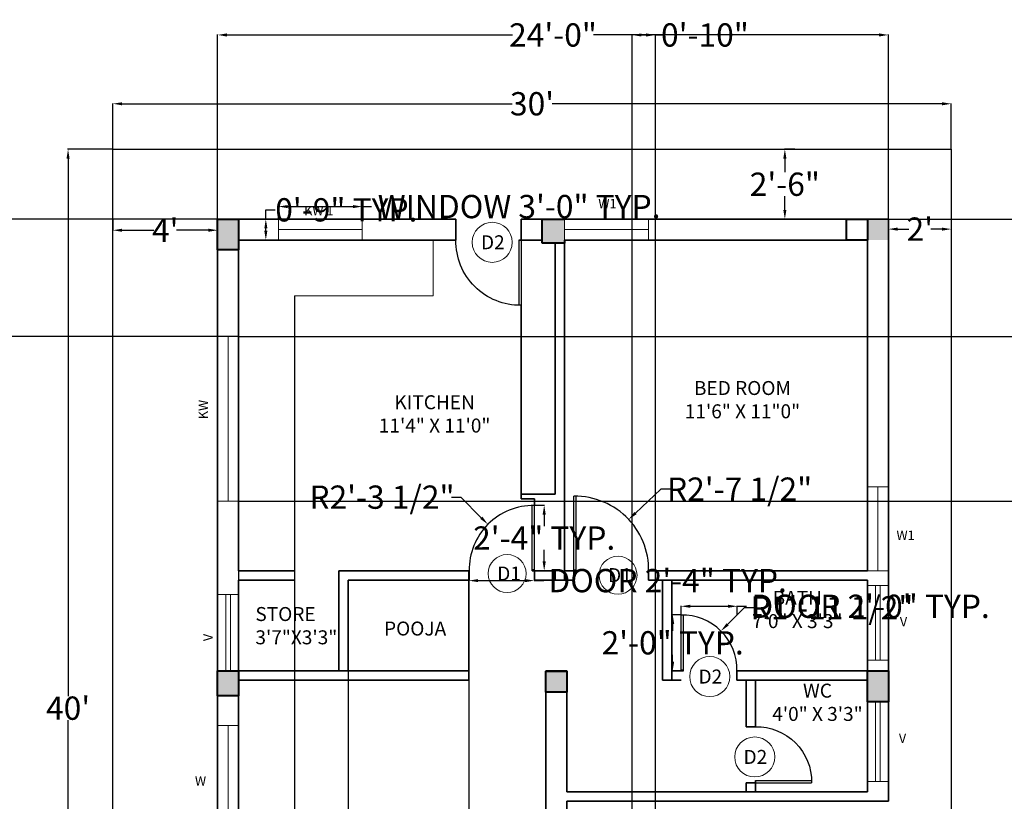
# Model space of a CAD drawing. Units: inches. Extents: x 529 to 1659, y 271 to 1222.
# Tile 4 of 5: x 936 to 1358, y 886 to 1222. Entities that reach past the tile are written whole.
import ezdxf

# ---------------------------------------------------------------- set-up
doc = ezdxf.new("R2010")
doc.units = ezdxf.units.IN
doc.header["$MEASUREMENT"] = 0
for name, color, linetype, lineweight in [('A-AREA-IDEN', 7, 'Continuous', 18), ('A-COLS', 7, 'Continuous', 40), ('A-COLS-PATT', 252, 'Continuous', 13), ('A-FLOR-FIXT', 8, 'Continuous', 18), ('COMPOUND WALL', 7, 'Continuous', 25), ('DIM', 241, 'Continuous', 18), ('DOOR', 4, 'Continuous', 25), ('TEXT', 131, 'Continuous', 18), ('VN', 3, 'Continuous', 18), ('WALL', 7, 'Continuous', 35), ('WDS', 4, 'Continuous', 18)]:
    doc.layers.add(name, color=color, linetype=linetype, lineweight=lineweight)
doc.styles.get("Standard").update_dxf_attribs({"font": 'arial.ttf', "height": 10})
doc.dimstyles.get("Standard").update_dxf_attribs({"dimtxt": 6, "dimasz": 4, "dimexe": 0.18, "dimexo": 0.0625, "dimgap": 0.09, "dimtad": 0, "dimtih": 1, "dimtoh": 1, "dimdec": 0, "dimrnd": 6, "dimzin": 0, "dimdsep": 46, "dimlunit": 3, "dimtxsty": 'Standard', "dimcen": 0.09, "dimadec": 0, "dimazin": 0, "dimtfac": 1, "dimtdec": 0, "dimtofl": 0, "dimtmove": 0, "dimatfit": 3, "dimfxl": 1, "dimtolj": 1, "dimtzin": 0, "dimarcsym": 0})

# ---------------------------------------------------------------- blocks, each defined once
blk = doc.blocks.new('*D1')
at = {"layer": 'Defpoints', "color": 0, "transparency": 16777216}
for p in [(1308.49, 1135.86), (1335.49, 1135.86), (1335.49, 1131.58)]:
    blk.add_point(p, dxfattribs=at)
at = {"layer": 'DIM', "color": 0, "lineweight": -2, "transparency": 16777216}
for p, q in [((1308.49, 1135.79), (1308.49, 1131.4)), ((1335.49, 1135.79), (1335.49, 1131.4)), ((1312.49, 1131.58), (1317.22, 1131.58)), ((1331.49, 1131.58), (1326.77, 1131.58))]:
    blk.add_line(p, q, dxfattribs=at)
at = {"layer": 'DIM', "color": 0, "transparency": 16777216}
for points in [[(1312.49, 1132.24), (1312.49, 1130.91), (1308.49, 1131.58)], [(1331.49, 1132.24), (1331.49, 1130.91), (1335.49, 1131.58)]]:
    blk.add_solid(points, dxfattribs=at)
at = {"layer": 'DIM', "color": 0, "transparency": 16777216, "insert": (1321.99, 1131.58), "char_height": 10, "attachment_point": 5}
blk.add_mtext("\\A1;2'", dxfattribs=at)
blk = doc.blocks.new('*D2')
at = {"layer": 'Defpoints', "color": 0, "transparency": 16777216}
for p in [(1264.05, 1165.86), (1268.35, 1165.86), (1268.35, 1135.86)]:
    blk.add_point(p, dxfattribs=at)
at = {"layer": 'DIM', "color": 0, "lineweight": -2, "transparency": 16777216}
for p, q in [((1268.28, 1165.86), (1263.87, 1165.86)), ((1264.05, 1161.86), (1264.05, 1156.05)), ((1264.05, 1139.86), (1264.05, 1145.66)), ((1268.28, 1135.86), (1263.87, 1135.86))]:
    blk.add_line(p, q, dxfattribs=at)
at = {"layer": 'DIM', "color": 0, "transparency": 16777216}
for points in [[(1263.38, 1161.86), (1264.72, 1161.86), (1264.05, 1165.86)], [(1263.38, 1139.86), (1264.72, 1139.86), (1264.05, 1135.86)]]:
    blk.add_solid(points, dxfattribs=at)
at = {"layer": 'DIM', "color": 0, "transparency": 16777216, "insert": (1264.05, 1150.86), "char_height": 10, "attachment_point": 5}
blk.add_mtext('\\A1;2\'-6"', dxfattribs=at)
blk = doc.blocks.new('*D3')
at = {"layer": 'Defpoints', "color": 0, "transparency": 16777216}
for p in [(975.49, 1135.86), (1020.49, 1135.86), (975.49, 1131.1)]:
    blk.add_point(p, dxfattribs=at)
at = {"layer": 'DIM', "color": 0, "lineweight": -2, "transparency": 16777216}
for p, q in [((975.49, 1135.79), (975.49, 1130.92)), ((1020.49, 1135.79), (1020.49, 1130.92)), ((979.49, 1131.1), (993.1, 1131.1)), ((1016.49, 1131.1), (1002.88, 1131.1))]:
    blk.add_line(p, q, dxfattribs=at)
at = {"layer": 'DIM', "color": 0, "transparency": 16777216}
for points in [[(979.49, 1131.77), (979.49, 1130.43), (975.49, 1131.1)], [(1016.49, 1131.77), (1016.49, 1130.43), (1020.49, 1131.1)]]:
    blk.add_solid(points, dxfattribs=at)
at = {"layer": 'DIM', "color": 0, "transparency": 16777216, "insert": (997.99, 1131.1), "char_height": 10, "attachment_point": 5}
blk.add_mtext("\\A1;4'", dxfattribs=at)
blk = doc.blocks.new('*D5')
at = {"layer": 'Defpoints', "color": 0, "transparency": 16777216}
for p in [(956.28, 1165.86), (975.49, 1165.86), (975.49, 685.86)]:
    blk.add_point(p, dxfattribs=at)
at = {"layer": 'DIM', "color": 0, "lineweight": -2, "transparency": 16777216}
for p, q in [((975.43, 1165.86), (956.1, 1165.86)), ((956.28, 1161.86), (956.28, 931.05)), ((956.28, 689.86), (956.28, 920.66)), ((975.43, 685.86), (956.1, 685.86))]:
    blk.add_line(p, q, dxfattribs=at)
at = {"layer": 'DIM', "color": 0, "transparency": 16777216}
for points in [[(955.61, 1161.86), (956.94, 1161.86), (956.28, 1165.86)], [(955.61, 689.86), (956.94, 689.86), (956.28, 685.86)]]:
    blk.add_solid(points, dxfattribs=at)
at = {"layer": 'DIM', "color": 0, "transparency": 16777216, "insert": (956.28, 925.86), "char_height": 10, "attachment_point": 5}
blk.add_mtext("\\A1;40'", dxfattribs=at)
blk = doc.blocks.new('*D6')
at = {"layer": 'Defpoints', "color": 0, "transparency": 16777216}
for p in [(1335.49, 1185.41), (975.49, 1165.86), (1335.49, 1165.86)]:
    blk.add_point(p, dxfattribs=at)
at = {"layer": 'DIM', "color": 0, "lineweight": -2, "transparency": 16777216}
for p, q in [((975.49, 1165.92), (975.49, 1185.59)), ((979.49, 1185.41), (1146.92, 1185.41)), ((1331.49, 1185.41), (1164.07, 1185.41)), ((1335.49, 1165.92), (1335.49, 1185.59))]:
    blk.add_line(p, q, dxfattribs=at)
at = {"layer": 'DIM', "color": 0, "transparency": 16777216}
for points in [[(979.49, 1186.07), (979.49, 1184.74), (975.49, 1185.41)], [(1331.49, 1186.07), (1331.49, 1184.74), (1335.49, 1185.41)]]:
    blk.add_solid(points, dxfattribs=at)
at = {"layer": 'DIM', "color": 0, "transparency": 16777216, "insert": (1155.49, 1185.41), "char_height": 10, "attachment_point": 5}
blk.add_mtext("\\A1;30'", dxfattribs=at)
blk = doc.blocks.new('DOOR-SWING-28IN')
for p, q in [((27, 0), (27, 28)), ((28, 0), (28, 28))]:
    blk.add_line(p, q)
blk.add_arc((27.5, 0.5), 27.5, 88.9584, 181.0416)
blk = doc.blocks.new('DOOR-SWING-24IN')
for p, q in [((0, 0), (0, 24)), ((1, 0), (1, 24))]:
    blk.add_line(p, q)
blk.add_arc((0.5, 0.5), 23.51, 358.7811, 91.2189)
blk = doc.blocks.new('WIN-36IN')
for p, q in [((0, 0), (0, 9)), ((36, 0), (36, 9)), ((36, 4.5), (0, 4.5))]:
    blk.add_line(p, q)
blk = doc.blocks.new('WIN-48IN')
for p, q in [((9, 48), (0, 48)), ((4.5, 0), (4.5, 48)), ((9, 0), (0, 0))]:
    blk.add_line(p, q)
blk = doc.blocks.new('COL-9X9IN')
blk.add_lwpolyline([(0, 9), (9, 9), (9, 0), (0, 0)], close=True)
blk = doc.blocks.new('DOOR-TAG-D1')
blk.add_circle((8.16, 8.16), 8.16)
at = {"insert": (3.9, 11.18), "char_height": 6, "attachment_point": 1}
blk.add_mtext_dynamic_manual_height_columns('D1', width=7.906, gutter_width=20, heights=[0], dxfattribs=at)
blk = doc.blocks.new('DOOR-TAG-D2')
blk.add_circle((8.6, 8.6), 8.6)
at = {"insert": (3.78, 11.61), "char_height": 6, "attachment_point": 1}
blk.add_mtext_dynamic_manual_height_columns('D2', width=7.906, gutter_width=20, heights=[0], dxfattribs=at)
blk = doc.blocks.new('*D19')
at = {"layer": 'Defpoints', "color": 0, "transparency": 16777216}
for p in [(1082.59, 1141.26), (1046.59, 1135.86), (1082.59, 1135.86)]:
    blk.add_point(p, dxfattribs=at)
at = {"layer": 'DIM', "color": 0, "lineweight": -2, "transparency": 16777216}
for p, q in [((1046.59, 1135.92), (1046.59, 1141.44)), ((1050.59, 1141.26), (1078.59, 1141.26)), ((1082.59, 1135.92), (1082.59, 1141.44)), ((1082.59, 1141.26), (1086.59, 1141.26))]:
    blk.add_line(p, q, dxfattribs=at)
at = {"layer": 'DIM', "color": 0, "transparency": 16777216}
for points in [[(1050.59, 1141.92), (1050.59, 1140.59), (1046.59, 1141.26)], [(1078.59, 1141.92), (1078.59, 1140.59), (1082.59, 1141.26)]]:
    blk.add_solid(points, dxfattribs=at)
at = {"layer": 'DIM', "color": 0, "transparency": 16777216, "insert": (1149.95, 1141.26), "char_height": 10, "attachment_point": 5}
blk.add_mtext('\\A1;WINDOW 3\'-0" TYP.', dxfattribs=at)
blk = doc.blocks.new('*D20')
at = {"layer": 'Defpoints', "color": 0, "transparency": 16777216}
for p in [(1041.19, 1135.86), (1046.59, 1135.86), (1046.59, 1126.86)]:
    blk.add_point(p, dxfattribs=at)
at = {"layer": 'DIM', "color": 0, "lineweight": -2, "transparency": 16777216}
for p, q in [((1041.19, 1135.86), (1041.19, 1139.86)), ((1041.19, 1139.86), (1045.19, 1139.86)), ((1046.53, 1135.86), (1041.01, 1135.86)), ((1041.19, 1130.86), (1041.19, 1131.86)), ((1046.53, 1126.86), (1041.01, 1126.86))]:
    blk.add_line(p, q, dxfattribs=at)
at = {"layer": 'DIM', "color": 0, "transparency": 16777216}
for points in [[(1040.53, 1131.86), (1041.86, 1131.86), (1041.19, 1135.86)], [(1040.53, 1130.86), (1041.86, 1130.86), (1041.19, 1126.86)]]:
    blk.add_solid(points, dxfattribs=at)
at = {"layer": 'DIM', "color": 0, "transparency": 16777216, "insert": (1075.76, 1139.86), "char_height": 10, "attachment_point": 5}
blk.add_mtext('\\A1;0\'-9" TYP.', dxfattribs=at)
blk = doc.blocks.new('*D23')
at = {"layer": 'Defpoints', "color": 0, "transparency": 16777216}
for p in [(1128.36, 984.86), (1156.49, 984.86), (1156.49, 980.63)]:
    blk.add_point(p, dxfattribs=at)
at = {"layer": 'DIM', "color": 0, "lineweight": -2, "transparency": 16777216}
for p, q in [((1128.36, 984.79), (1128.36, 980.45)), ((1156.49, 984.79), (1156.49, 980.45)), ((1132.36, 980.63), (1152.49, 980.63)), ((1156.49, 980.63), (1160.49, 980.63))]:
    blk.add_line(p, q, dxfattribs=at)
at = {"layer": 'DIM', "color": 0, "transparency": 16777216}
for points in [[(1132.36, 981.3), (1132.36, 979.97), (1128.36, 980.63)], [(1152.49, 981.3), (1152.49, 979.97), (1156.49, 980.63)]]:
    blk.add_solid(points, dxfattribs=at)
at = {"layer": 'DIM', "color": 0, "transparency": 16777216, "insert": (1213.71, 980.63), "char_height": 10, "attachment_point": 5}
blk.add_mtext('\\A1;DOOR 2\'-4" TYP.', dxfattribs=at)
blk = doc.blocks.new('*D24')
at = {"layer": 'Defpoints', "color": 0, "transparency": 16777216}
for p in [(1156.49, 1012.99), (1160.71, 1012.99), (1156.49, 984.86)]:
    blk.add_point(p, dxfattribs=at)
at = {"layer": 'DIM', "color": 0, "lineweight": -2, "transparency": 16777216}
for p, q in [((1156.56, 1012.99), (1160.89, 1012.99)), ((1160.71, 1008.99), (1160.71, 1004.04)), ((1160.71, 988.86), (1160.71, 993.81)), ((1156.56, 984.86), (1160.89, 984.86))]:
    blk.add_line(p, q, dxfattribs=at)
at = {"layer": 'DIM', "color": 0, "transparency": 16777216}
for points in [[(1160.05, 1008.99), (1161.38, 1008.99), (1160.71, 1012.99)], [(1160.05, 988.86), (1161.38, 988.86), (1160.71, 984.86)]]:
    blk.add_solid(points, dxfattribs=at)
at = {"layer": 'DIM', "color": 0, "transparency": 16777216, "insert": (1160.71, 998.92), "char_height": 10, "attachment_point": 5}
blk.add_mtext('\\A1;2\'-4" TYP.', dxfattribs=at)
blk = doc.blocks.new('*D25')
at = {"layer": 'Defpoints', "color": 0, "transparency": 16777216}
for p in [(1243.63, 969.61), (1219.49, 965.99), (1243.63, 965.99)]:
    blk.add_point(p, dxfattribs=at)
at = {"layer": 'DIM', "color": 0, "lineweight": -2, "transparency": 16777216}
for p, q in [((1219.49, 966.05), (1219.49, 969.79)), ((1223.49, 969.61), (1239.63, 969.61)), ((1243.63, 966.05), (1243.63, 969.79)), ((1243.63, 969.61), (1247.63, 969.61))]:
    blk.add_line(p, q, dxfattribs=at)
at = {"layer": 'DIM', "color": 0, "transparency": 16777216}
for points in [[(1223.49, 970.28), (1223.49, 968.95), (1219.49, 969.61)], [(1239.63, 970.28), (1239.63, 968.95), (1243.63, 969.61)]]:
    blk.add_solid(points, dxfattribs=at)
at = {"layer": 'DIM', "color": 0, "transparency": 16777216, "insert": (1300.84, 969.61), "char_height": 10, "attachment_point": 5}
blk.add_mtext('\\A1;DOOR 2\'-0" TYP.', dxfattribs=at)
blk = doc.blocks.new('*D26')
at = {"layer": 'Defpoints', "color": 0, "transparency": 16777216}
for p in [(1215.87, 965.99), (1219.49, 965.99), (1219.49, 941.86)]:
    blk.add_point(p, dxfattribs=at)
at = {"layer": 'DIM', "color": 0, "lineweight": -2, "transparency": 16777216}
for p, q in [((1219.43, 965.99), (1215.69, 965.99)), ((1215.87, 961.99), (1215.87, 959.12)), ((1215.87, 945.86), (1215.87, 948.73)), ((1219.43, 941.86), (1215.69, 941.86))]:
    blk.add_line(p, q, dxfattribs=at)
at = {"layer": 'DIM', "color": 0, "transparency": 16777216}
for points in [[(1215.21, 961.99), (1216.54, 961.99), (1215.87, 965.99)], [(1215.21, 945.86), (1216.54, 945.86), (1215.87, 941.86)]]:
    blk.add_solid(points, dxfattribs=at)
at = {"layer": 'DIM', "color": 0, "transparency": 16777216, "insert": (1215.87, 953.92), "char_height": 10, "attachment_point": 5}
blk.add_mtext('\\A1;2\'-0" TYP.', dxfattribs=at)
blk = doc.blocks.new('*D27')
at = {"layer": 'Defpoints', "color": 0, "transparency": 16777216}
for p in [(1308.49, 1214.96), (1020.49, 1135.86), (1308.49, 1135.86)]:
    blk.add_point(p, dxfattribs=at)
at = {"layer": 'DIM', "color": 0, "lineweight": -2, "transparency": 16777216}
for p, q in [((1020.49, 1135.92), (1020.49, 1215.14)), ((1024.49, 1214.96), (1147.14, 1214.96)), ((1304.49, 1214.96), (1181.84, 1214.96)), ((1308.49, 1135.92), (1308.49, 1215.14))]:
    blk.add_line(p, q, dxfattribs=at)
at = {"layer": 'DIM', "color": 0, "transparency": 16777216}
for points in [[(1024.49, 1215.62), (1024.49, 1214.29), (1020.49, 1214.96)], [(1304.49, 1215.62), (1304.49, 1214.29), (1308.49, 1214.96)]]:
    blk.add_solid(points, dxfattribs=at)
at = {"layer": 'DIM', "color": 0, "transparency": 16777216, "insert": (1164.49, 1214.96), "char_height": 10, "attachment_point": 5}
blk.add_mtext('\\A1;24\'-0"', dxfattribs=at)
blk = doc.blocks.new('*D28')
at = {"layer": 'Defpoints', "color": 0, "transparency": 16777216}
for p in [(1308.49, 1135.86), (1630, 1135.86), (1308.49, 685.86)]:
    blk.add_point(p, dxfattribs=at)
at = {"layer": 'DIM', "color": 0, "lineweight": -2, "transparency": 16777216}
for p, q in [((1308.56, 1135.86), (1630.18, 1135.86)), ((1630, 1131.86), (1630, 916.05)), ((1630, 689.86), (1630, 905.66)), ((1308.56, 685.86), (1630.18, 685.86))]:
    blk.add_line(p, q, dxfattribs=at)
at = {"layer": 'DIM', "color": 0, "transparency": 16777216}
for points in [[(1629.34, 1131.86), (1630.67, 1131.86), (1630, 1135.86)], [(1629.34, 689.86), (1630.67, 689.86), (1630, 685.86)]]:
    blk.add_solid(points, dxfattribs=at)
at = {"layer": 'DIM', "color": 0, "transparency": 16777216, "insert": (1630, 910.86), "char_height": 10, "attachment_point": 5}
blk.add_mtext('\\A1;37\'-6"', dxfattribs=at)
blk = doc.blocks.new('*D29')
at = {"layer": 'Defpoints', "color": 0, "transparency": 16777216}
for p in [(1076.49, 941.86), (1128.41, 941.86), (1128.41, 277.14)]:
    blk.add_point(p, dxfattribs=at)
at = {"layer": 'DIM', "color": 0, "lineweight": -2, "transparency": 16777216}
for p, q in [((1076.49, 941.79), (1076.49, 276.96)), ((1128.41, 941.79), (1128.41, 276.96)), ((1080.49, 277.14), (1088.87, 277.14)), ((1124.41, 277.14), (1116.04, 277.14))]:
    blk.add_line(p, q, dxfattribs=at)
at = {"layer": 'DIM', "color": 0, "transparency": 16777216}
for points in [[(1080.49, 277.81), (1080.49, 276.47), (1076.49, 277.14)], [(1124.41, 277.81), (1124.41, 276.47), (1128.41, 277.14)]]:
    blk.add_solid(points, dxfattribs=at)
at = {"layer": 'DIM', "color": 0, "transparency": 16777216, "insert": (1102.45, 277.14), "char_height": 10, "attachment_point": 5}
blk.add_mtext('\\A1;4\'-4"', dxfattribs=at)
blk = doc.blocks.new('*D34')
at = {"layer": 'Defpoints', "color": 0, "transparency": 16777216}
for p in [(1029.49, 1085.43), (1630, 1085.43), (1029.49, 1014.68)]:
    blk.add_point(p, dxfattribs=at)
at = {"layer": 'DIM', "color": 0, "lineweight": -2, "transparency": 16777216}
for p, q in [((1029.56, 1085.43), (1630.18, 1085.43)), ((1630, 1081.43), (1630, 1055.32)), ((1630, 1018.68), (1630, 1044.8)), ((1029.56, 1014.68), (1630.18, 1014.68))]:
    blk.add_line(p, q, dxfattribs=at)
at = {"layer": 'DIM', "color": 0, "transparency": 16777216}
for points in [[(1629.34, 1081.43), (1630.67, 1081.43), (1630, 1085.43)], [(1629.34, 1018.68), (1630.67, 1018.68), (1630, 1014.68)]]:
    blk.add_solid(points, dxfattribs=at)
at = {"layer": 'DIM', "color": 0, "transparency": 16777216, "insert": (1630, 1050.06), "char_height": 10, "attachment_point": 5}
blk.add_mtext('\\A1;5\'-10 1/2"', dxfattribs=at)
blk = doc.blocks.new('*D35')
at = {"layer": 'Defpoints', "color": 0, "transparency": 16777216}
for p in [(555.49, 1135.86), (1020.49, 1135.86), (1029.49, 1085.43)]:
    blk.add_point(p, dxfattribs=at)
at = {"layer": 'DIM', "color": 0, "lineweight": -2, "transparency": 16777216}
for p, q in [((1020.43, 1135.86), (555.31, 1135.86)), ((555.49, 1131.86), (555.49, 1115.9)), ((555.49, 1089.43), (555.49, 1105.38)), ((1029.43, 1085.43), (555.31, 1085.43))]:
    blk.add_line(p, q, dxfattribs=at)
at = {"layer": 'DIM', "color": 0, "transparency": 16777216}
for points in [[(554.83, 1131.86), (556.16, 1131.86), (555.49, 1135.86)], [(554.83, 1089.43), (556.16, 1089.43), (555.49, 1085.43)]]:
    blk.add_solid(points, dxfattribs=at)
at = {"layer": 'DIM', "color": 0, "transparency": 16777216, "insert": (555.49, 1110.64), "char_height": 10, "attachment_point": 5}
blk.add_mtext('\\A1;4\'-2 1/2"', dxfattribs=at)
blk = doc.blocks.new('*D36')
at = {"layer": 'Defpoints', "color": 0, "transparency": 16777216}
for p in [(1029.49, 1126.86), (1053.49, 1102.86), (1053.49, 277.14)]:
    blk.add_point(p, dxfattribs=at)
at = {"layer": 'DIM', "color": 0, "lineweight": -2, "transparency": 16777216}
for p, q in [((1029.49, 1126.79), (1029.49, 276.96)), ((1053.49, 1102.79), (1053.49, 276.96)), ((1033.49, 277.14), (1049.49, 277.14)), ((1053.49, 277.14), (1057.49, 277.14))]:
    blk.add_line(p, q, dxfattribs=at)
at = {"layer": 'DIM', "color": 0, "transparency": 16777216}
for points in [[(1033.49, 277.81), (1033.49, 276.47), (1029.49, 277.14)], [(1049.49, 277.81), (1049.49, 276.47), (1053.49, 277.14)]]:
    blk.add_solid(points, dxfattribs=at)
at = {"layer": 'DIM', "color": 0, "transparency": 16777216, "insert": (1070.96, 277.14), "char_height": 10, "attachment_point": 5}
blk.add_mtext('\\A1;2\'-0"', dxfattribs=at)
blk = doc.blocks.new('*D37')
at = {"layer": 'Defpoints', "color": 0, "transparency": 16777216}
for p in [(1208.47, 1214.96), (1198.47, 826.86), (1208.47, 826.86)]:
    blk.add_point(p, dxfattribs=at)
at = {"layer": 'DIM', "color": 0, "lineweight": -2, "transparency": 16777216}
for p, q in [((1198.47, 826.92), (1198.47, 1215.14)), ((1202.47, 1214.96), (1204.47, 1214.96)), ((1208.47, 826.92), (1208.47, 1215.14)), ((1208.47, 1214.96), (1212.47, 1214.96))]:
    blk.add_line(p, q, dxfattribs=at)
at = {"layer": 'DIM', "color": 0, "transparency": 16777216}
for points in [[(1202.47, 1215.62), (1202.47, 1214.29), (1198.47, 1214.96)], [(1204.47, 1215.62), (1204.47, 1214.29), (1208.47, 1214.96)]]:
    blk.add_solid(points, dxfattribs=at)
at = {"layer": 'DIM', "color": 0, "transparency": 16777216, "insert": (1229.74, 1214.96), "char_height": 10, "attachment_point": 5}
blk.add_mtext('\\A1;0\'-10"', dxfattribs=at)
blk = doc.blocks.new('*D38')
at = {"layer": 'Defpoints', "color": 0, "transparency": 16777216}
for p in [(1197, 1006.92), (1173.99, 985.27)]:
    blk.add_point(p, dxfattribs=at)
at = {"layer": 'DIM', "color": 0, "lineweight": -2, "transparency": 16777216}
for p, q in [((1210.8, 1019.91), (1199.91, 1009.66)), ((1214.8, 1019.91), (1210.8, 1019.91)), ((1173.9, 985.27), (1174.08, 985.27)), ((1173.99, 985.18), (1173.99, 985.36))]:
    blk.add_line(p, q, dxfattribs=at)
at = {"layer": 'DIM', "color": 0, "transparency": 16777216}
blk.add_solid([(1199.45, 1010.15), (1200.37, 1009.18), (1197, 1006.92)], dxfattribs=at)
at = {"layer": 'DIM', "color": 0, "transparency": 16777216, "insert": (1244.62, 1019.91), "char_height": 10, "attachment_point": 5}
blk.add_mtext('\\A1;R2\'-7 1/2"', dxfattribs=at)
blk = doc.blocks.new('*D39')
at = {"layer": 'Defpoints', "color": 0, "transparency": 16777216}
for p in [(1136.54, 1004.8), (1155.99, 985.36)]:
    blk.add_point(p, dxfattribs=at)
at = {"layer": 'DIM', "color": 0, "lineweight": -2, "transparency": 16777216}
for p, q in [((1120.87, 1016.47), (1124.87, 1016.47)), ((1124.87, 1016.47), (1133.72, 1007.63)), ((1155.9, 985.36), (1156.08, 985.36)), ((1155.99, 985.27), (1155.99, 985.45))]:
    blk.add_line(p, q, dxfattribs=at)
at = {"layer": 'DIM', "color": 0, "transparency": 16777216}
blk.add_solid([(1134.19, 1008.1), (1133.24, 1007.16), (1136.54, 1004.8)], dxfattribs=at)
at = {"layer": 'DIM', "color": 0, "transparency": 16777216, "insert": (1091.06, 1016.47), "char_height": 10, "attachment_point": 5}
blk.add_mtext('\\A1;R2\'-3 1/2"', dxfattribs=at)
blk = doc.blocks.new('*D40')
at = {"layer": 'Defpoints', "color": 0, "transparency": 16777216}
for p in [(1236.61, 958.98), (1219.99, 942.36)]:
    blk.add_point(p, dxfattribs=at)
at = {"layer": 'DIM', "color": 0, "lineweight": -2, "transparency": 16777216}
for p, q in [((1246.59, 968.95), (1239.44, 961.8)), ((1250.59, 968.95), (1246.59, 968.95)), ((1219.9, 942.36), (1220.08, 942.36)), ((1219.99, 942.27), (1219.99, 942.45))]:
    blk.add_line(p, q, dxfattribs=at)
at = {"layer": 'DIM', "color": 0, "transparency": 16777216}
blk.add_solid([(1238.97, 962.28), (1239.91, 961.33), (1236.61, 958.98)], dxfattribs=at)
at = {"layer": 'DIM', "color": 0, "transparency": 16777216, "insert": (1284.29, 968.95), "char_height": 10, "attachment_point": 5}
blk.add_mtext('\\A1;R1\'-11 1/2"', dxfattribs=at)

msp = doc.modelspace()

# ---------------------------------------------------------------- hatches: boundary and pattern name
at = {"layer": 'A-COLS-PATT'}
h = msp.add_hatch(color=256, dxfattribs=at)
h.dxf.hatch_style = 1
h.paths.add_polyline_path([(1169.49, 1135.86), (1159.82, 1135.86), (1159.82, 1125.57), (1169.49, 1125.57), (1169.49, 1126.86)])
h.paths.add_polyline_path([(1308.49, 1135.86), (1299.49, 1135.86), (1299.49, 1126.86), (1308.49, 1126.86)])
h.paths.add_polyline_path([(1029.49, 1135.86), (1020.49, 1135.86), (1020.49, 1122.62), (1029.49, 1122.62)])
h.paths.add_polyline_path([(1029.49, 941.86), (1020.49, 941.86), (1020.49, 931.16), (1029.49, 931.16)])
h.paths.add_polyline_path([(1170.49, 941.72), (1161.49, 941.72), (1161.49, 932.72), (1170.49, 932.72)])
h.paths.add_polyline_path([(1308.49, 941.86), (1299.49, 941.86), (1299.49, 928.64), (1308.49, 928.64)])
h.paths.add_polyline_path([(1308.49, 826.86), (1299.49, 826.86), (1299.49, 817.86), (1308.49, 817.86)])
h.paths.add_polyline_path([(1170.49, 826.93), (1161.49, 826.93), (1161.49, 817.93), (1170.49, 817.93)])
h.paths.add_polyline_path([(1308.49, 706.86), (1299.49, 706.86), (1299.49, 697.86), (1308.49, 697.86)])
h.paths.add_polyline_path([(1170.49, 706.86), (1161.49, 706.86), (1161.49, 697.86), (1170.49, 697.86)])
h.paths.add_polyline_path([(1029.41, 750.01), (1020.49, 750.01), (1020.49, 736.86), (1029.49, 736.86)])

# ---------------------------------------------------------------- linework, layer by layer
at = {"layer": 'A-COLS'}
for p, q in [((1159.82, 1125.57), (1159.82, 1135.86)), ((1159.82, 1135.86), (1169.49, 1135.86)), ((1169.49, 1125.57), (1159.82, 1125.57)), ((1169.49, 1126.86), (1169.49, 1125.57)), ((1020.49, 931.16), (1020.49, 941.86)), ((1020.49, 941.86), (1029.49, 941.86)), ((1029.49, 941.86), (1029.49, 931.16)), ((1299.49, 941.86), (1308.49, 941.86)), ((1299.49, 928.64), (1299.49, 941.86)), ((1308.49, 941.86), (1308.49, 928.64)), ((1029.49, 931.16), (1020.49, 931.16)), ((1308.49, 928.64), (1299.49, 928.64))]:
    msp.add_line(p, q, dxfattribs=at)
msp.add_lwpolyline([(1020.49, 1135.86), (1029.49, 1135.86), (1029.49, 1122.62), (1020.49, 1122.62)], close=True, dxfattribs=at)
at = {"layer": 'A-FLOR-FIXT'}
for p, q in [((1113.1, 1126.86), (1113.1, 1102.86)), ((1053.49, 980.86), (1053.49, 1102.86)), ((1053.49, 1102.86), (1113.1, 1102.86))]:
    msp.add_line(p, q, dxfattribs=at)
at = {"layer": 'COMPOUND WALL'}
for p, q in [((975.49, 1165.86), (1335.49, 1165.86)), ((975.49, 685.86), (975.49, 1165.86)), ((1335.49, 1165.86), (1335.49, 685.86))]:
    msp.add_line(p, q, dxfattribs=at)
at = {"layer": 'DOOR'}
for p, q in [((1173.49, 984.86), (1173.49, 1016.86)), ((1174.49, 984.86), (1174.49, 1016.86))]:
    msp.add_line(p, q, dxfattribs=at)
msp.add_arc((1173.99, 985.27), 31.59, 355.6218, 90.9068, dxfattribs=at)
at = {"layer": 'VN'}
for p, q in [((1299.49, 978.49), (1308.49, 978.49)), ((1302.99, 946.49), (1302.99, 978.49)), ((1304.99, 946.49), (1304.99, 978.49)), ((1029.49, 974.65), (1020.49, 974.65)), ((1023.99, 941.86), (1023.99, 974.65)), ((1025.99, 941.86), (1025.99, 974.65)), ((1299.49, 946.49), (1308.49, 946.49)), ((1302.99, 894.38), (1302.99, 928.64)), ((1304.99, 894.38), (1304.99, 928.64)), ((1308.49, 894.38), (1299.49, 894.38))]:
    msp.add_line(p, q, dxfattribs=at)
at = {"layer": 'WALL'}
for p, q in [((1020.49, 1135.86), (1122.82, 1135.86)), ((1020.49, 697.86), (1020.49, 1135.86)), ((1122.82, 1126.86), (1122.82, 1135.86)), ((1150.82, 1126.86), (1150.82, 1135.86)), ((1150.82, 1135.86), (1308.49, 1135.86)), ((1308.49, 1135.86), (1308.49, 885.86)), ((1308.49, 1135.86), (1308.49, 885.86)), ((1029.49, 1126.86), (1122.82, 1126.86)), ((1029.49, 984.86), (1029.49, 1126.86)), ((1149.82, 1126.86), (1159.82, 1126.86)), ((1165.49, 1017.73), (1165.49, 1125.57)), ((1169.49, 1126.86), (1299.49, 1126.86)), ((1169.49, 984.86), (1169.49, 1126.86)), ((1299.49, 1126.86), (1299.49, 984.86)), ((1150.82, 1098.86), (1150.82, 1015.73)), ((1165.49, 1017.73), (1150.82, 1017.73)), ((1156.49, 1015.73), (1150.82, 1015.73)), ((1156.49, 1012.86), (1156.49, 1015.73)), ((1029.49, 984.86), (1053.49, 984.86)), ((1029.49, 980.86), (1053.49, 980.86)), ((1029.49, 736.86), (1029.49, 980.86)), ((1072.49, 941.86), (1072.49, 984.86)), ((1072.49, 984.86), (1128.49, 984.86)), ((1076.49, 941.86), (1076.49, 980.86)), ((1076.49, 980.86), (1128.49, 980.86)), ((1128.41, 937.86), (1128.41, 984.86)), ((1128.49, 980.86), (1128.49, 984.86)), ((1155.49, 984.86), (1165.49, 984.86)), ((1156.49, 980.86), (1156.49, 984.86)), ((1156.49, 980.86), (1173.49, 980.86)), ((1165.49, 980.86), (1165.49, 984.86)), ((1169.49, 980.86), (1169.49, 984.86)), ((1169.49, 984.86), (1174.49, 984.86)), ((1173.49, 980.86), (1173.49, 984.86)), ((1205.49, 980.86), (1205.49, 984.86)), ((1205.49, 984.86), (1299.49, 984.86)), ((1205.49, 980.86), (1299.49, 980.86)), ((1211.49, 980.86), (1211.49, 937.86)), ((1215.49, 980.86), (1215.49, 937.86)), ((1299.49, 980.86), (1299.49, 889.86)), ((1029.49, 941.86), (1072.49, 941.86)), ((1029.49, 941.86), (1128.41, 941.86)), ((1029.49, 941.86), (1121.07, 941.86)), ((1161.49, 736.86), (1161.49, 941.86)), ((1161.49, 941.86), (1170.49, 941.86)), ((1161.49, 941.86), (1170.49, 941.86)), ((1170.49, 889.86), (1170.49, 941.86)), ((1215.49, 941.86), (1220.49, 941.86)), ((1243.49, 941.86), (1243.49, 937.86)), ((1243.49, 941.86), (1299.49, 941.86)), ((1029.49, 937.86), (1128.41, 937.86)), ((1211.49, 937.86), (1219.49, 937.86)), ((1243.49, 937.86), (1299.49, 937.86)), ((1247.49, 937.86), (1247.49, 917.86)), ((1251.49, 937.86), (1251.49, 917.86)), ((1247.49, 917.86), (1251.49, 917.86)), ((1247.49, 893.86), (1251.49, 893.86)), ((1247.49, 893.86), (1247.49, 889.86)), ((1251.49, 894.86), (1251.49, 889.86)), ((1170.49, 889.86), (1247.49, 889.86)), ((1247.49, 889.86), (1299.49, 889.86)), ((1170.49, 885.86), (1308.49, 885.86)), ((1170.49, 826.86), (1170.49, 885.86))]:
    msp.add_line(p, q, dxfattribs=at)
at = {"layer": 'WDS'}
for p, q in [((1029.49, 1085.43), (1020.49, 1085.43)), ((1024.99, 1014.68), (1024.99, 1085.43)), ((1029.49, 1014.68), (1020.49, 1014.68))]:
    msp.add_line(p, q, dxfattribs=at)

# ---------------------------------------------------------------- block references
at = {"layer": 'A-COLS'}
for p in [(1290.49, 1126.86), (1161.49, 932.72)]:
    msp.add_blockref('COL-9X9IN', p, dxfattribs=at)
at = {"layer": 'DOOR', "extrusion": (0, 0, -1), "zscale": -1}
for name, p, rotation in [('DOOR-SWING-28IN', (-1122.82, 1126.86), 180), ('DOOR-SWING-24IN', (-1251.49, 893.86), 89.99999999999989)]:
    msp.add_blockref(name, p, dxfattribs=dict(at, rotation=rotation))
at = {"layer": 'DOOR'}
for name, p in [('DOOR-SWING-28IN', (1128.49, 984.86)), ('DOOR-SWING-24IN', (1219.49, 941.85))]:
    msp.add_blockref(name, p, dxfattribs=at)
at = {"layer": 'TEXT'}
for name, p in [('DOOR-TAG-D2', (1129.79, 1117.31)), ('DOOR-TAG-D1', (1136.64, 975.5)), ('DOOR-TAG-D1', (1184.26, 974.8)), ('DOOR-TAG-D2', (1223.2, 930.82)), ('DOOR-TAG-D2', (1242.53, 896.3))]:
    msp.add_blockref(name, p, dxfattribs=at)
at = {"layer": 'WDS'}
for name, p in [('WIN-36IN', (1046.59, 1126.86)), ('WIN-48IN', (1020.49, 870.43))]:
    msp.add_blockref(name, p, dxfattribs=at)
for p, rotation in [((1205.49, 1135.86), 180), ((1308.49, 984.86), 89.99999999999974)]:
    msp.add_blockref('WIN-36IN', p, dxfattribs=dict(at, rotation=rotation))

# ---------------------------------------------------------------- texts
at = {"layer": 'A-AREA-IDEN', "attachment_point": 1}
for s, width, insert, char_height in [('\\pxqc;BED ROOM\\P11\'6" X 11"0"', 60.9783, (1215.36, 1066.34), 6), ('\\pxqc;KITCHEN\\P11\'4" X 11\'0"', 48.0168, (1089.66, 1060.23), 6), ('\\pxqc;BATH\\P7\'0" X 3\'3"', 50.606, (1244.09, 976.24), 6), ('{\\H1.5x;STORE\\P3\'7"X3\'3"}  ', 18.1132, (1036.71, 969.28), 4), ('POOJA', 27.5467, (1091.95, 963.05), 6), ('\\pxqc;WC\\P4\'0" X 3\'3"', 48.1384, (1253.98, 936.38), 6)]:
    msp.add_mtext_dynamic_manual_height_columns(s, width=width, gutter_width=20, heights=[0], dxfattribs=dict(at, insert=insert, char_height=char_height))
at = {"layer": 'TEXT', "char_height": 4, "attachment_point": 1}
for s, width, insert in [('\\pxqc;KW 1', 22.8322, (1052.51, 1141.56)), ('W1 ', 22.0133, (1183.96, 1144.54)), ('W1 ', 22.0133, (1311.97, 1002.12)), ('V ', 39.464, (1313.01, 914.94)), ('W ', 22.0133, (1010.76, 896.57))]:
    msp.add_mtext_dynamic_manual_height_columns(s, width=width, gutter_width=20, heights=[0], dxfattribs=dict(at, insert=insert))
for s, width, insert, rotation in [('\\pxqc;KW  ', 22.8322, (1012.29, 1042.7), 90), ('V ', 39.464, (1313.42, 964.96), 1.046), ('V ', 39.464, (1014.35, 954.62), 90)]:
    msp.add_mtext_dynamic_manual_height_columns(s, width=width, gutter_width=20, heights=[0], dxfattribs=dict(at, insert=insert, rotation=rotation))

# ---------------------------------------------------------------- dimensions: what is measured, and where the dimension line sits
at = {"layer": 'DIM'}
for base, p1, p2, override, picture, middle in [((1308.49, 1214.96), (1020.49, 1135.86), (1308.49, 1135.86), {"dimdec": 1, "dimlfac": 1, "dimrnd": 0, "dimzin": 1, "dimdsep": 46, "dimlunit": 4, "dimfrac": 2}, '*D27', (1164.49, 1214.96)), ((1208.47, 1214.96), (1198.47, 826.86), (1208.47, 826.86), {"dimdec": 1, "dimlfac": 1, "dimrnd": 0, "dimzin": 1, "dimdsep": 46, "dimlunit": 4, "dimfrac": 2}, '*D37', (1229.74, 1214.96)), ((1335.49, 1185.41), (975.49, 1165.86), (1335.49, 1165.86), {"dimclrd": 0, "dimclre": 0, "dimclrt": 0}, '*D6', (1155.49, 1185.41)), ((975.49, 1131.1), (1020.49, 1135.86), (975.49, 1135.86), {"dimclrd": 0, "dimclre": 0, "dimclrt": 0}, '*D3', (997.99, 1131.1)), ((1335.49, 1131.58), (1308.49, 1135.86), (1335.49, 1135.86), {"dimclrd": 0, "dimclre": 0, "dimclrt": 0}, '*D1', (1321.99, 1131.58)), ((1053.49, 277.14), (1029.49, 1126.86), (1053.49, 1102.86), {"dimdec": 1, "dimlfac": 1, "dimrnd": 0, "dimzin": 1, "dimdsep": 46, "dimlunit": 4, "dimfrac": 2}, '*D36', (1070.96, 277.14)), ((1128.41, 277.14), (1076.49, 941.86), (1128.41, 941.86), {"dimdec": 1, "dimlfac": 1, "dimrnd": 0, "dimzin": 1, "dimdsep": 46, "dimlunit": 4, "dimfrac": 2}, '*D29', (1102.45, 277.14))]:
    dim = msp.add_linear_dim(base=base, p1=p1, p2=p2, dimstyle='Standard', override=override, dxfattribs=at)
    dim.commit()
    dim.dimension.update_dxf_attribs({"geometry": picture, "text_midpoint": middle})
for base, p1, p2, override, picture, middle in [((956.28, 1165.86), (975.49, 685.86), (975.49, 1165.86), {"dimclrd": 0, "dimclre": 0, "dimclrt": 0}, '*D5', (956.28, 925.86)), ((1264.05, 1165.86), (1268.35, 1135.86), (1268.35, 1165.86), {"dimclrd": 0, "dimclre": 0, "dimclrt": 0}, '*D2', (1264.05, 1150.86)), ((555.49, 1135.86), (1029.49, 1085.43), (1020.49, 1135.86), {"dimdec": 1, "dimlfac": 1, "dimrnd": 0, "dimzin": 1, "dimdsep": 46, "dimlunit": 4, "dimfrac": 2}, '*D35', (555.49, 1110.64)), ((1630, 1135.86), (1308.49, 685.86), (1308.49, 1135.86), {"dimdec": 1, "dimlfac": 1, "dimrnd": 0, "dimzin": 1, "dimdsep": 46, "dimlunit": 4, "dimfrac": 2}, '*D28', (1630, 910.86)), ((1630.0017, 1085.4304), (1029.4928, 1014.6812), (1029.4928, 1085.4304), {"dimdec": 1, "dimlfac": 1, "dimrnd": 0, "dimzin": 1, "dimdsep": 46, "dimlunit": 4, "dimfrac": 2}, '*D34', (1630.0017, 1050.0558))]:
    dim = msp.add_linear_dim(base=base, p1=p1, p2=p2, angle=90, dimstyle='Standard', override=override, dxfattribs=at)
    dim.commit()
    dim.dimension.update_dxf_attribs({"geometry": picture, "text_midpoint": middle})
for base, p1, p2, text, picture, middle in [((1082.59, 1141.26), (1046.59, 1135.86), (1082.59, 1135.86), 'WINDOW <> TYP.', '*D19', (1149.95, 1141.26)), ((1156.49, 980.63), (1128.36, 984.86), (1156.49, 984.86), 'DOOR <> TYP.', '*D23', (1213.71, 980.63)), ((1243.63, 969.61), (1219.49, 965.99), (1243.63, 965.99), 'DOOR <> TYP.', '*D25', (1300.84, 969.61))]:
    dim = msp.add_linear_dim(base=base, p1=p1, p2=p2, text=text, dimstyle='Standard', override={"dimdec": 1, "dimlfac": 1, "dimrnd": 0, "dimzin": 1, "dimdsep": 46, "dimlunit": 4, "dimfrac": 2}, dxfattribs=at)
    dim.commit()
    dim.dimension.update_dxf_attribs({"geometry": picture, "text_midpoint": middle})
for base, p1, p2, picture, middle in [((1041.19, 1135.86), (1046.59, 1126.86), (1046.59, 1135.86), '*D20', (1075.76, 1139.86)), ((1160.71, 1012.99), (1156.49, 984.86), (1156.49, 1012.99), '*D24', (1160.71, 998.92)), ((1215.87, 965.99), (1219.49, 941.86), (1219.49, 965.99), '*D26', (1215.87, 953.92))]:
    dim = msp.add_linear_dim(base=base, p1=p1, p2=p2, angle=90, text='<> TYP.', dimstyle='Standard', override={"dimdec": 1, "dimlfac": 1, "dimrnd": 0, "dimzin": 1, "dimdsep": 46, "dimlunit": 4, "dimfrac": 2}, dxfattribs=at)
    dim.commit()
    dim.dimension.update_dxf_attribs({"geometry": picture, "text_midpoint": middle})
for center, mpoint, picture, middle in [((1173.99, 985.27), (1197, 1006.92), '*D38', (1244.62, 1019.91)), ((1155.99, 985.36), (1136.54, 1004.8), '*D39', (1091.06, 1016.47)), ((1219.99, 942.36), (1236.61, 958.98), '*D40', (1284.29, 968.95))]:
    dim = msp.add_radius_dim(center=center, mpoint=mpoint, dimstyle='Standard', override={"dimdec": 1, "dimlfac": 1, "dimrnd": 0, "dimzin": 1, "dimdsep": 46, "dimlunit": 4, "dimfrac": 2}, dxfattribs=at)
    dim.commit()
    dim.dimension.update_dxf_attribs({"geometry": picture, "text_midpoint": middle, "dimtype": 164})

doc.saveas('drawing.dxf')
